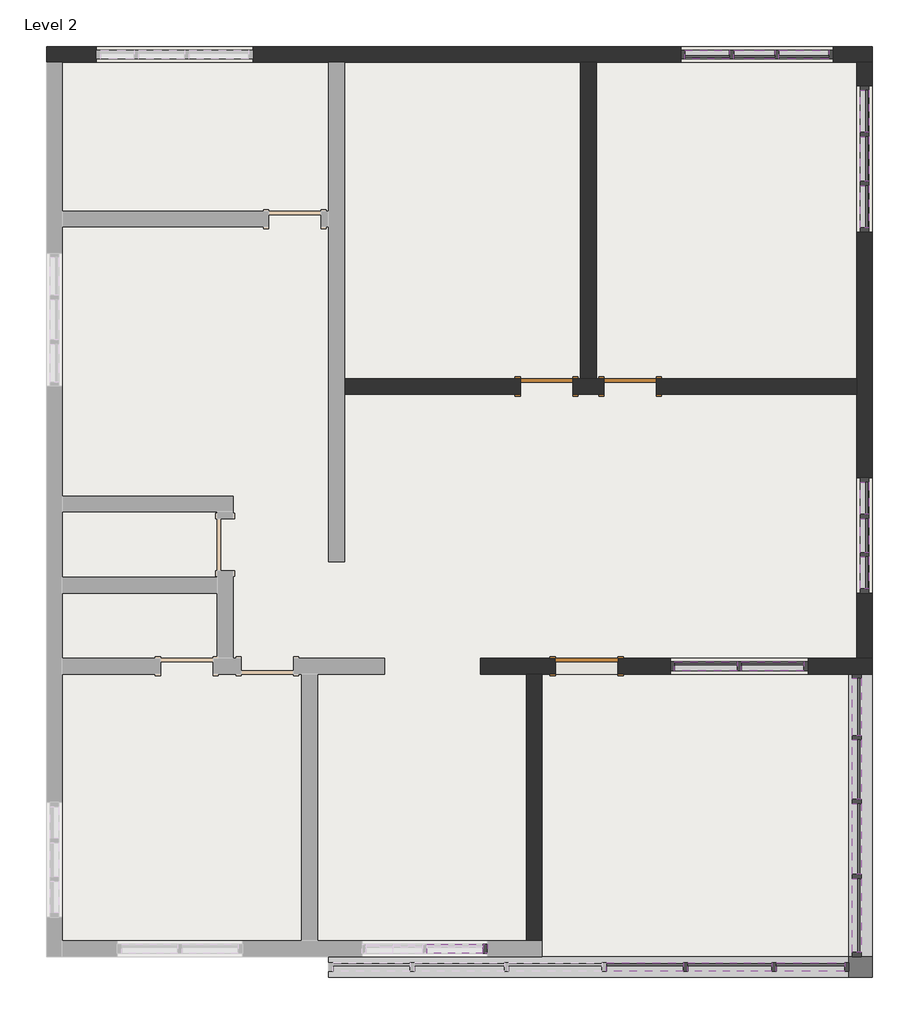
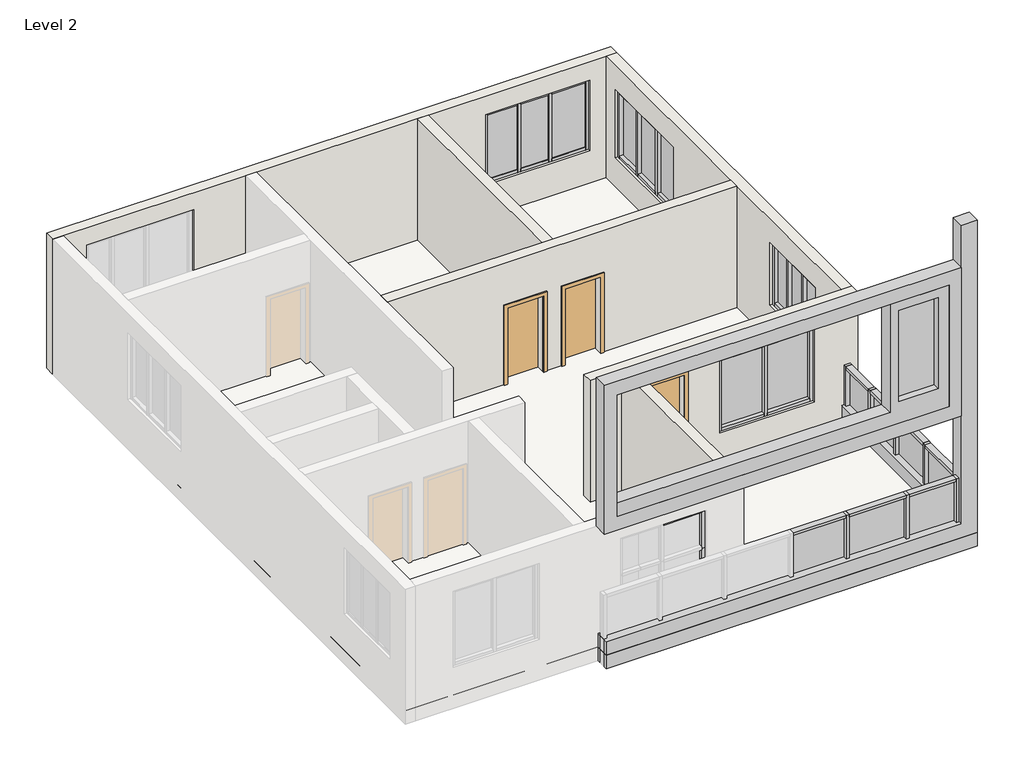
# One storey, part 2 of 2: 59 members, 18 plates, 6 walls, 3 doors, 2 proxies, 1 roof.
"""IFC4 building model written with IfcOpenShell, lengths in millimetres."""

from ifc_helpers import new_model, si_unit, frame, origin, place, context, project, spatial, polyline, outline, extrude, faceted_brep, transform, mapped, element, save
from components import generic_models_2_generic_models_2_cc0d390d, generic_models_3_generic_models_3_7314e451, door_a1484949, door_85036156, door_a90ba1ad, member_3f0e0172, member_5215b92c, member_61359a5b, member_c17f1be2, member_5535eeb3, member_2ebf4a73, member_0bf31a60, member_647c50ce, member_78a9872f, member_43b5e5be, member_a400357f, member_ea9411ea, member_8d44de84, member_42ca508f, member_8c3e4394, member_cac0d47b, member_4a65ca8f, member_0adfe7f4, member_001188f2, member_75b26f99, member_883d71fc, member_d722639b, member_62e0d4bf, member_79ceace6, member_4d6ef9b1, member_b70ee1cc, member_c5864796, member_66f327b8, member_a80f276a, system_panel_glazed_83e43f9b, system_panel_glazed_4ceb7c04, system_panel_glazed_bbfcf774, system_panel_glazed_f5702331, system_panel_glazed_135d4218, system_panel_glazed_d2b782c8, system_panel_glazed_c0907c48, system_panel_glazed_aa593011, system_panel_glazed_fc0c7c09, system_panel_glazed_9bd642df, system_panel_glazed_a16c717b, system_panel_glazed_1cb891c7, system_panel_glazed_caa91b16, system_panel_glazed_a6fb9a4f, system_panel_glazed_64bca335

model = new_model("IFC4")

# Units and contexts
model_context = context("Model", 3, world=origin())
ifc_project = project(units=[si_unit("LENGTHUNIT", "METRE", prefix="MILLI")], contexts=[model_context])

# Site, building, storey
site = spatial("IfcSite", under=ifc_project)
building = spatial("IfcBuilding", under=site)
storey = spatial("IfcBuildingStorey", under=building, Name="Level 2", Elevation=3048.0)

# Proxies
placement = place(None, origin())
generic_models_2_generic_models_2_shape = generic_models_2_generic_models_2_cc0d390d(model_context)
element("IfcBuildingElementProxy", 1, Name="Generic Models 2 : Generic Models 2", ObjectType="Generic Models 2 : Generic Models 2", at=placement, inside=storey, context=model_context, shape_type="MappedRepresentation", body=[
    mapped(generic_models_2_generic_models_2_shape, transform((0.0, 0.0, 0.0), x_axis=(1.0, 0.0, 0.0), y_axis=(0.0, 1.0, 0.0), z_axis=(0.0, 0.0, 1.0))),
])
generic_models_3_generic_models_3_shape = generic_models_3_generic_models_3_7314e451(model_context)
element("IfcBuildingElementProxy", 2, Name="Generic Models 3 : Generic Models 3", ObjectType="Generic Models 3 : Generic Models 3", at=placement, inside=storey, context=model_context, shape_type="MappedRepresentation", body=[
    mapped(generic_models_3_generic_models_3_shape, transform((0.0, 0.0, 0.0), x_axis=(1.0, 0.0, 0.0), y_axis=(0.0, 1.0, 0.0), z_axis=(0.0, 0.0, 1.0))),
])

# Doors
door_shape = door_a1484949(model_context)
element("IfcDoor", 3, ObjectType="Single-Flush : 30\" x 80\"", at=placement, inside=storey, context=model_context, shape_type="MappedRepresentation", body=[
    mapped(door_shape, transform((-12995.791855, -5548.3538163, 3048.0), x_axis=(1.0, 0.0, 0.0), y_axis=(0.0, 1.0, 0.0), z_axis=(0.0, 0.0, 1.0))),
])
door_2_shape = door_85036156(model_context)
element("IfcDoor", 4, ObjectType="Single-Flush : 30\" x 80\"", at=placement, inside=storey, context=model_context, shape_type="MappedRepresentation", body=[
    mapped(door_2_shape, transform((-11776.591855, -5548.3538163, 3048.0), x_axis=(-1.0, 0.0, 0.0), y_axis=(0.0, -1.0, 0.0), z_axis=(0.0, 0.0, 1.0))),
])
door_3_shape = door_a90ba1ad(model_context)
element("IfcDoor", 5, ObjectType="Single-Flush : 36\" x 84\"", at=placement, inside=storey, context=model_context, shape_type="MappedRepresentation", body=[
    mapped(door_3_shape, transform((-12411.591855, -9625.0538163, 3403.6), x_axis=(-1.0, 0.0, 0.0), y_axis=(0.0, -1.0, 0.0), z_axis=(0.0, 0.0, 1.0))),
])

# Members
member_shape = member_3f0e0172(model_context)
element("IfcMember", 6, ObjectType="Rectangular Mullion : 2.5\" x 5\" rectangular", at=placement, inside=storey, context=model_context, shape_type="MappedRepresentation", body=[
    mapped(member_shape, transform((-8360.291855, -2621.0038163, 4007.4850468), x_axis=(0.0, 0.0, -1.0), y_axis=(-1.0, 0.0, 0.0), z_axis=(0.0, 1.0, 0.0))),
])
element("IfcMember", 7, ObjectType="Rectangular Mullion : 2.5\" x 5\" rectangular", at=placement, inside=storey, context=model_context, shape_type="MappedRepresentation", body=[
    mapped(member_shape, transform((-8360.291855, -1230.3538163, 4007.4850468), x_axis=(0.0, 0.0, -1.0), y_axis=(-1.0, 0.0, 0.0), z_axis=(0.0, 1.0, 0.0))),
])
member_2_shape = member_5215b92c(model_context)
element("IfcMember", 8, ObjectType="Rectangular Mullion : 2.5\" x 5\" rectangular", at=placement, inside=storey, context=model_context, shape_type="MappedRepresentation", body=[
    mapped(member_2_shape, transform((-8360.291855, -1909.8038163, 4007.4850468), x_axis=(0.0, 0.0, -1.0), y_axis=(-1.0, 0.0, 0.0), z_axis=(0.0, 1.0, 0.0))),
])
element("IfcMember", 9, ObjectType="Rectangular Mullion : 2.5\" x 5\" rectangular", at=placement, inside=storey, context=model_context, shape_type="MappedRepresentation", body=[
    mapped(member_2_shape, transform((-8360.291855, -2557.5038163, 5545.6790625), x_axis=(0.0, 0.0, 1.0), y_axis=(-1.0, 0.0, 0.0), z_axis=(0.0, -1.0, 0.0))),
])
element("IfcMember", 10, ObjectType="Rectangular Mullion : 2.5\" x 5\" rectangular", at=placement, inside=storey, context=model_context, shape_type="MappedRepresentation", body=[
    mapped(member_shape, transform((-8360.291855, -1846.3038163, 5545.6790625), x_axis=(0.0, 0.0, 1.0), y_axis=(-1.0, 0.0, 0.0), z_axis=(0.0, -1.0, 0.0))),
])
element("IfcMember", 11, ObjectType="Rectangular Mullion : 2.5\" x 5\" rectangular", at=placement, inside=storey, context=model_context, shape_type="MappedRepresentation", body=[
    mapped(member_shape, transform((-8360.291855, -3236.9538163, 5545.6790625), x_axis=(0.0, 0.0, 1.0), y_axis=(-1.0, 0.0, 0.0), z_axis=(0.0, -1.0, 0.0))),
])
member_3_shape = member_61359a5b(model_context)
element("IfcMember", 12, ObjectType="Rectangular Mullion : 2.5\" x 5\" rectangular", at=placement, inside=storey, context=model_context, shape_type="MappedRepresentation", body=[
    mapped(member_3_shape, transform((-10976.491855, -709.6538163, 5669.9128008), x_axis=(0.0, 0.0, 1.0), y_axis=(0.0, 1.0, 0.0), z_axis=(-1.0, 0.0, 0.0))),
])
element("IfcMember", 13, ObjectType="Rectangular Mullion : 2.5\" x 5\" rectangular", at=placement, inside=storey, context=model_context, shape_type="MappedRepresentation", body=[
    mapped(member_3_shape, transform((-10330.9085217, -709.6538163, 4085.5528144), x_axis=(0.0, 0.0, -1.0), y_axis=(0.0, 1.0, 0.0), z_axis=(1.0, 0.0, 0.0))),
])
member_4_shape = member_c17f1be2(model_context)
element("IfcMember", 14, ObjectType="Rectangular Mullion : 2.5\" x 5\" rectangular", at=placement, inside=storey, context=model_context, shape_type="MappedRepresentation", body=[
    mapped(member_4_shape, transform((-13922.891855, -13739.8538163, 5631.310527), x_axis=(0.0, 0.0, 1.0), y_axis=(0.0, -1.0, 0.0), z_axis=(1.0, 0.0, 0.0))),
])
member_5_shape = member_5535eeb3(model_context)
element("IfcMember", 15, ObjectType="Rectangular Mullion : 2.5\" x 5\" rectangular", at=placement, inside=storey, context=model_context, shape_type="MappedRepresentation", body=[
    mapped(member_5_shape, transform((-8360.291855, -7408.9038163, 5557.0770518), x_axis=(0.0, 0.0, 1.0), y_axis=(-1.0, 0.0, 0.0), z_axis=(0.0, -1.0, 0.0))),
])
element("IfcMember", 16, ObjectType="Rectangular Mullion : 2.5\" x 5\" rectangular", at=placement, inside=storey, context=model_context, shape_type="MappedRepresentation", body=[
    mapped(member_5_shape, transform((-8360.291855, -8494.7538163, 5557.0770518), x_axis=(0.0, 0.0, 1.0), y_axis=(-1.0, 0.0, 0.0), z_axis=(0.0, -1.0, 0.0))),
])
member_6_shape = member_2ebf4a73(model_context)
element("IfcMember", 17, ObjectType="Rectangular Mullion : 2.5\" x 5\" rectangular", at=placement, inside=storey, context=model_context, shape_type="MappedRepresentation", body=[
    mapped(member_6_shape, transform((-8360.291855, -7967.7038163, 5557.0770518), x_axis=(0.0, 0.0, 1.0), y_axis=(-1.0, 0.0, 0.0), z_axis=(0.0, -1.0, 0.0))),
])
member_7_shape = member_0bf31a60(model_context)
element("IfcMember", 18, ObjectType="Rectangular Mullion : 2.5\" x 5\" rectangular", at=placement, inside=storey, context=model_context, shape_type="MappedRepresentation", body=[
    mapped(member_7_shape, transform((-8360.291855, -7440.6538163, 4148.8893788), x_axis=(0.0, -1.0, 0.0), y_axis=(-1.0, 0.0, 0.0), z_axis=(0.0, 0.0, -1.0))),
])
element("IfcMember", 19, ObjectType="Rectangular Mullion : 2.5\" x 5\" rectangular", at=placement, inside=storey, context=model_context, shape_type="MappedRepresentation", body=[
    mapped(member_7_shape, transform((-8360.291855, -7999.4538163, 4148.8893788), x_axis=(0.0, -1.0, 0.0), y_axis=(-1.0, 0.0, 0.0), z_axis=(0.0, 0.0, -1.0))),
])
element("IfcMember", 20, ObjectType="Rectangular Mullion : 2.5\" x 5\" rectangular", at=placement, inside=storey, context=model_context, shape_type="MappedRepresentation", body=[
    mapped(member_6_shape, transform((-8360.291855, -7472.4038163, 4148.8893788), x_axis=(0.0, 0.0, -1.0), y_axis=(-1.0, 0.0, 0.0), z_axis=(0.0, 1.0, 0.0))),
])
element("IfcMember", 21, ObjectType="Rectangular Mullion : 2.5\" x 5\" rectangular", at=placement, inside=storey, context=model_context, shape_type="MappedRepresentation", body=[
    mapped(member_5_shape, transform((-8360.291855, -8031.2038163, 4148.8893788), x_axis=(0.0, 0.0, -1.0), y_axis=(-1.0, 0.0, 0.0), z_axis=(0.0, 1.0, 0.0))),
])
element("IfcMember", 22, ObjectType="Rectangular Mullion : 2.5\" x 5\" rectangular", at=placement, inside=storey, context=model_context, shape_type="MappedRepresentation", body=[
    mapped(member_5_shape, transform((-8360.291855, -6945.3538163, 4148.8893788), x_axis=(0.0, 0.0, -1.0), y_axis=(-1.0, 0.0, 0.0), z_axis=(0.0, 1.0, 0.0))),
])
member_8_shape = member_647c50ce(model_context)
element("IfcMember", 23, ObjectType="Rectangular Mullion : 2.5\" x 5\" rectangular", at=placement, inside=storey, context=model_context, shape_type="MappedRepresentation", body=[
    mapped(member_8_shape, transform((-8360.291855, -6881.8538163, 5557.0770518), x_axis=(0.0, 1.0, 0.0), y_axis=(-1.0, 0.0, 0.0), z_axis=(0.0, 0.0, 1.0))),
])
element("IfcMember", 24, ObjectType="Rectangular Mullion : 2.5\" x 5\" rectangular", at=placement, inside=storey, context=model_context, shape_type="MappedRepresentation", body=[
    mapped(member_8_shape, transform((-8360.291855, -8558.2538163, 4148.8893788), x_axis=(0.0, -1.0, 0.0), y_axis=(-1.0, 0.0, 0.0), z_axis=(0.0, 0.0, -1.0))),
])
member_9_shape = member_78a9872f(model_context)
element("IfcMember", 25, ObjectType="Rectangular Mullion : 2.5\" x 5\" rectangular", at=placement, inside=storey, context=model_context, shape_type="MappedRepresentation", body=[
    mapped(member_9_shape, transform((-8360.291855, -1878.0538163, 4007.4850468), x_axis=(0.0, -1.0, 0.0), y_axis=(-1.0, 0.0, 0.0), z_axis=(0.0, 0.0, -1.0))),
])
element("IfcMember", 26, ObjectType="Rectangular Mullion : 2.5\" x 5\" rectangular", at=placement, inside=storey, context=model_context, shape_type="MappedRepresentation", body=[
    mapped(member_9_shape, transform((-8360.291855, -2589.2538163, 4007.4850468), x_axis=(0.0, -1.0, 0.0), y_axis=(-1.0, 0.0, 0.0), z_axis=(0.0, 0.0, -1.0))),
])
member_10_shape = member_43b5e5be(model_context)
element("IfcMember", 27, ObjectType="Rectangular Mullion : 2.5\" x 5\" rectangular", at=placement, inside=storey, context=model_context, shape_type="MappedRepresentation", body=[
    mapped(member_10_shape, transform((-8360.291855, -1166.8538163, 5545.6790625), x_axis=(0.0, 1.0, 0.0), y_axis=(-1.0, 0.0, 0.0), z_axis=(0.0, 0.0, 1.0))),
])
element("IfcMember", 28, ObjectType="Rectangular Mullion : 2.5\" x 5\" rectangular", at=placement, inside=storey, context=model_context, shape_type="MappedRepresentation", body=[
    mapped(member_10_shape, transform((-8360.291855, -3300.4538163, 4007.4850468), x_axis=(0.0, -1.0, 0.0), y_axis=(-1.0, 0.0, 0.0), z_axis=(0.0, 0.0, -1.0))),
])
member_11_shape = member_a400357f(model_context)
element("IfcMember", 29, ObjectType="Rectangular Mullion : 2.5\" x 5\" rectangular", at=placement, inside=storey, context=model_context, shape_type="MappedRepresentation", body=[
    mapped(member_11_shape, transform((-9670.5085217, -709.6538163, 4085.5528144), x_axis=(0.0, 0.0, -1.0), y_axis=(0.0, 1.0, 0.0), z_axis=(1.0, 0.0, 0.0))),
])
member_12_shape = member_ea9411ea(model_context)
element("IfcMember", 30, ObjectType="Rectangular Mullion : 2.5\" x 5\" rectangular", at=placement, inside=storey, context=model_context, shape_type="MappedRepresentation", body=[
    mapped(member_12_shape, transform((-8880.991855, -709.6538163, 4085.5528144), x_axis=(0.0, 0.0, -1.0), y_axis=(0.0, 1.0, 0.0), z_axis=(1.0, 0.0, 0.0))),
])
member_13_shape = member_8d44de84(model_context)
element("IfcMember", 31, ObjectType="Rectangular Mullion : 2.5\" x 5\" rectangular", at=placement, inside=storey, context=model_context, shape_type="MappedRepresentation", body=[
    mapped(member_13_shape, transform((-10299.1585217, -709.6538163, 4085.5528144), x_axis=(-1.0, 0.0, 0.0), y_axis=(0.0, 1.0, 0.0), z_axis=(0.0, 0.0, -1.0))),
])
element("IfcMember", 32, ObjectType="Rectangular Mullion : 2.5\" x 5\" rectangular", at=placement, inside=storey, context=model_context, shape_type="MappedRepresentation", body=[
    mapped(member_13_shape, transform((-9638.7585217, -709.6538163, 4085.5528144), x_axis=(-1.0, 0.0, 0.0), y_axis=(0.0, 1.0, 0.0), z_axis=(0.0, 0.0, -1.0))),
])
element("IfcMember", 33, ObjectType="Rectangular Mullion : 2.5\" x 5\" rectangular", at=placement, inside=storey, context=model_context, shape_type="MappedRepresentation", body=[
    mapped(member_12_shape, transform((-9607.0085217, -709.6538163, 5669.9128008), x_axis=(0.0, 0.0, 1.0), y_axis=(0.0, 1.0, 0.0), z_axis=(-1.0, 0.0, 0.0))),
])
element("IfcMember", 34, ObjectType="Rectangular Mullion : 2.5\" x 5\" rectangular", at=placement, inside=storey, context=model_context, shape_type="MappedRepresentation", body=[
    mapped(member_11_shape, transform((-10267.4085217, -709.6538163, 5669.9128008), x_axis=(0.0, 0.0, 1.0), y_axis=(0.0, 1.0, 0.0), z_axis=(-1.0, 0.0, 0.0))),
])
member_14_shape = member_42ca508f(model_context)
element("IfcMember", 35, ObjectType="Rectangular Mullion : 2.5\" x 5\" rectangular", at=placement, inside=storey, context=model_context, shape_type="MappedRepresentation", body=[
    mapped(member_14_shape, transform((-11039.991855, -709.6538163, 4085.5528144), x_axis=(-1.0, 0.0, 0.0), y_axis=(0.0, 1.0, 0.0), z_axis=(0.0, 0.0, -1.0))),
])
element("IfcMember", 36, ObjectType="Rectangular Mullion : 2.5\" x 5\" rectangular", at=placement, inside=storey, context=model_context, shape_type="MappedRepresentation", body=[
    mapped(member_14_shape, transform((-8817.491855, -709.6538163, 5669.9128008), x_axis=(1.0, 0.0, 0.0), y_axis=(0.0, 1.0, 0.0), z_axis=(0.0, 0.0, 1.0))),
])
member_15_shape = member_8c3e4394(model_context)
element("IfcMember", 37, ObjectType="Rectangular Mullion : 2.5\" x 5\" rectangular", at=placement, inside=storey, context=model_context, shape_type="MappedRepresentation", body=[
    mapped(member_15_shape, transform((-10217.666855, -9625.0538163, 5592.5131116), x_axis=(0.0, 0.0, 1.0), y_axis=(0.0, -1.0, 0.0), z_axis=(1.0, 0.0, 0.0))),
])
element("IfcMember", 38, ObjectType="Rectangular Mullion : 2.5\" x 5\" rectangular", at=placement, inside=storey, context=model_context, shape_type="MappedRepresentation", body=[
    mapped(member_15_shape, transform((-9242.941855, -9625.0538163, 5592.5131116), x_axis=(0.0, 0.0, 1.0), y_axis=(0.0, -1.0, 0.0), z_axis=(1.0, 0.0, 0.0))),
])
member_16_shape = member_cac0d47b(model_context)
element("IfcMember", 39, ObjectType="Rectangular Mullion : 2.5\" x 5\" rectangular", at=placement, inside=storey, context=model_context, shape_type="MappedRepresentation", body=[
    mapped(member_16_shape, transform((-10185.916855, -9625.0538163, 3942.9226891), x_axis=(1.0, 0.0, 0.0), y_axis=(0.0, -1.0, 0.0), z_axis=(0.0, 0.0, -1.0))),
])
element("IfcMember", 40, ObjectType="Rectangular Mullion : 2.5\" x 5\" rectangular", at=placement, inside=storey, context=model_context, shape_type="MappedRepresentation", body=[
    mapped(member_15_shape, transform((-10154.166855, -9625.0538163, 3942.9226891), x_axis=(0.0, 0.0, -1.0), y_axis=(0.0, -1.0, 0.0), z_axis=(-1.0, 0.0, 0.0))),
])
element("IfcMember", 41, ObjectType="Rectangular Mullion : 2.5\" x 5\" rectangular", at=placement, inside=storey, context=model_context, shape_type="MappedRepresentation", body=[
    mapped(member_15_shape, transform((-11128.891855, -9625.0538163, 3942.9226891), x_axis=(0.0, 0.0, -1.0), y_axis=(0.0, -1.0, 0.0), z_axis=(-1.0, 0.0, 0.0))),
])
member_17_shape = member_4a65ca8f(model_context)
element("IfcMember", 42, ObjectType="Rectangular Mullion : 2.5\" x 5\" rectangular", at=placement, inside=storey, context=model_context, shape_type="MappedRepresentation", body=[
    mapped(member_17_shape, transform((-9179.441855, -9625.0538163, 3942.9226891), x_axis=(1.0, 0.0, 0.0), y_axis=(0.0, -1.0, 0.0), z_axis=(0.0, 0.0, -1.0))),
])
element("IfcMember", 43, ObjectType="Rectangular Mullion : 2.5\" x 5\" rectangular", at=placement, inside=storey, context=model_context, shape_type="MappedRepresentation", body=[
    mapped(member_17_shape, transform((-11192.391855, -9625.0538163, 5592.5131116), x_axis=(-1.0, 0.0, 0.0), y_axis=(0.0, -1.0, 0.0), z_axis=(0.0, 0.0, 1.0))),
])
member_18_shape = member_0adfe7f4(model_context)
element("IfcMember", 44, ObjectType="Rectangular Mullion : 2.5\" x 5\" rectangular", at=placement, inside=storey, context=model_context, shape_type="MappedRepresentation", body=[
    mapped(member_18_shape, transform((-13859.391855, -13739.8538163, 4760.0253323), x_axis=(1.0, 0.0, 0.0), y_axis=(0.0, -1.0, 0.0), z_axis=(0.0, 0.0, -1.0))),
])
element("IfcMember", 45, ObjectType="Rectangular Mullion : 2.5\" x 5\" rectangular", at=placement, inside=storey, context=model_context, shape_type="MappedRepresentation", body=[
    mapped(member_18_shape, transform((-13859.391855, -13739.8538163, 3888.7401376), x_axis=(1.0, 0.0, 0.0), y_axis=(0.0, -1.0, 0.0), z_axis=(0.0, 0.0, -1.0))),
])
member_19_shape = member_001188f2(model_context)
element("IfcMember", 46, ObjectType="Rectangular Mullion : 2.5\" x 5\" rectangular", at=placement, inside=storey, context=model_context, shape_type="MappedRepresentation", body=[
    mapped(member_19_shape, transform((-9679.0607234, -14006.5538163, 3048.0), x_axis=(1.0, 0.0, 0.0), y_axis=(0.0, -1.0, 0.0), z_axis=(0.0, 0.0, -1.0))),
])
element("IfcMember", 47, ObjectType="Rectangular Mullion : 2.5\" x 5\" rectangular", at=placement, inside=storey, context=model_context, shape_type="MappedRepresentation", body=[
    mapped(member_19_shape, transform((-10967.3481445, -14006.5538163, 3048.0), x_axis=(1.0, 0.0, 0.0), y_axis=(0.0, -1.0, 0.0), z_axis=(0.0, 0.0, -1.0))),
])
member_20_shape = member_75b26f99(model_context)
element("IfcMember", 48, ObjectType="Rectangular Mullion : 2.5\" x 5\" rectangular", at=placement, inside=storey, context=model_context, shape_type="MappedRepresentation", body=[
    mapped(member_20_shape, transform((-8586.8607234, -14006.5538163, 3048.0), x_axis=(1.0, 0.0, 0.0), y_axis=(0.0, -1.0, 0.0), z_axis=(0.0, 0.0, -1.0))),
])
member_21_shape = member_883d71fc(model_context)
element("IfcMember", 49, ObjectType="Rectangular Mullion : 2.5\" x 5\" rectangular", at=placement, inside=storey, context=model_context, shape_type="MappedRepresentation", body=[
    mapped(member_21_shape, transform((-8650.3607234, -14006.5538163, 4647.2829369), x_axis=(0.0, 0.0, 1.0), y_axis=(0.0, -1.0, 0.0), z_axis=(1.0, 0.0, 0.0))),
])
member_22_shape = member_d722639b(model_context)
element("IfcMember", 50, ObjectType="Rectangular Mullion : 2.5\" x 5\" rectangular", at=placement, inside=storey, context=model_context, shape_type="MappedRepresentation", body=[
    mapped(member_22_shape, transform((-9710.8107234, -14006.5538163, 4647.2829369), x_axis=(0.0, 0.0, 1.0), y_axis=(0.0, -1.0, 0.0), z_axis=(1.0, 0.0, 0.0))),
])
member_23_shape = member_62e0d4bf(model_context)
element("IfcMember", 51, ObjectType="Rectangular Mullion : 2.5\" x 5\" rectangular", at=placement, inside=storey, context=model_context, shape_type="MappedRepresentation", body=[
    mapped(member_23_shape, transform((-10999.0981445, -14006.5538163, 4647.2829369), x_axis=(0.0, 0.0, 1.0), y_axis=(0.0, -1.0, 0.0), z_axis=(1.0, 0.0, 0.0))),
])
member_24_shape = member_79ceace6(model_context)
element("IfcMember", 52, ObjectType="Rectangular Mullion : 2.5\" x 5\" rectangular", at=placement, inside=storey, context=model_context, shape_type="MappedRepresentation", body=[
    mapped(member_24_shape, transform((-8474.591855, -11625.3038163, 3575.4206061), x_axis=(0.0, 0.0, -1.0), y_axis=(-1.0, 0.0, 0.0), z_axis=(0.0, 1.0, 0.0))),
])
member_25_shape = member_4d6ef9b1(model_context)
element("IfcMember", 53, ObjectType="Rectangular Mullion : 2.5\" x 5\" rectangular", at=placement, inside=storey, context=model_context, shape_type="MappedRepresentation", body=[
    mapped(member_25_shape, transform((-8474.591855, -12717.5038163, 3575.4206061), x_axis=(0.0, 0.0, -1.0), y_axis=(-1.0, 0.0, 0.0), z_axis=(0.0, 1.0, 0.0))),
])
member_26_shape = member_b70ee1cc(model_context)
element("IfcMember", 54, ObjectType="Rectangular Mullion : 2.5\" x 5\" rectangular", at=placement, inside=storey, context=model_context, shape_type="MappedRepresentation", body=[
    mapped(member_26_shape, transform((-8474.591855, -10698.2038163, 3575.4206061), x_axis=(0.0, 0.0, -1.0), y_axis=(-1.0, 0.0, 0.0), z_axis=(0.0, 1.0, 0.0))),
])
member_27_shape = member_c5864796(model_context)
element("IfcMember", 55, ObjectType="Rectangular Mullion : 2.5\" x 5\" rectangular", at=placement, inside=storey, context=model_context, shape_type="MappedRepresentation", body=[
    mapped(member_27_shape, transform((-8474.591855, -9802.8538163, 3575.4206061), x_axis=(0.0, 0.0, -1.0), y_axis=(-1.0, 0.0, 0.0), z_axis=(0.0, 1.0, 0.0))),
])
member_28_shape = member_66f327b8(model_context)
element("IfcMember", 56, ObjectType="Rectangular Mullion : 2.5\" x 5\" rectangular", at=placement, inside=storey, context=model_context, shape_type="MappedRepresentation", body=[
    mapped(member_28_shape, transform((-8474.591855, -12685.7538163, 3575.4206061), x_axis=(0.0, -1.0, 0.0), y_axis=(-1.0, 0.0, 0.0), z_axis=(0.0, 0.0, -1.0))),
])
element("IfcMember", 57, ObjectType="Rectangular Mullion : 2.5\" x 5\" rectangular", at=placement, inside=storey, context=model_context, shape_type="MappedRepresentation", body=[
    mapped(member_28_shape, transform((-8474.591855, -11593.5538163, 3575.4206061), x_axis=(0.0, -1.0, 0.0), y_axis=(-1.0, 0.0, 0.0), z_axis=(0.0, 0.0, -1.0))),
])
element("IfcMember", 58, ObjectType="Rectangular Mullion : 2.5\" x 5\" rectangular", at=placement, inside=storey, context=model_context, shape_type="MappedRepresentation", body=[
    mapped(member_28_shape, transform((-8474.591855, -10666.4538163, 3575.4206061), x_axis=(0.0, -1.0, 0.0), y_axis=(-1.0, 0.0, 0.0), z_axis=(0.0, 0.0, -1.0))),
])
element("IfcMember", 59, ObjectType="Rectangular Mullion : 2.5\" x 5\" rectangular", at=placement, inside=storey, context=model_context, shape_type="MappedRepresentation", body=[
    mapped(member_27_shape, transform((-8474.591855, -10634.7038163, 4555.4351711), x_axis=(0.0, 0.0, 1.0), y_axis=(-1.0, 0.0, 0.0), z_axis=(0.0, -1.0, 0.0))),
])
element("IfcMember", 60, ObjectType="Rectangular Mullion : 2.5\" x 5\" rectangular", at=placement, inside=storey, context=model_context, shape_type="MappedRepresentation", body=[
    mapped(member_26_shape, transform((-8474.591855, -11561.8038163, 4555.4351711), x_axis=(0.0, 0.0, 1.0), y_axis=(-1.0, 0.0, 0.0), z_axis=(0.0, -1.0, 0.0))),
])
element("IfcMember", 61, ObjectType="Rectangular Mullion : 2.5\" x 5\" rectangular", at=placement, inside=storey, context=model_context, shape_type="MappedRepresentation", body=[
    mapped(member_24_shape, transform((-8474.591855, -12654.0038163, 4555.4351711), x_axis=(0.0, 0.0, 1.0), y_axis=(-1.0, 0.0, 0.0), z_axis=(0.0, -1.0, 0.0))),
])
element("IfcMember", 62, ObjectType="Rectangular Mullion : 2.5\" x 5\" rectangular", at=placement, inside=storey, context=model_context, shape_type="MappedRepresentation", body=[
    mapped(member_25_shape, transform((-8474.591855, -13790.6538163, 4555.4351711), x_axis=(0.0, 0.0, 1.0), y_axis=(-1.0, 0.0, 0.0), z_axis=(0.0, -1.0, 0.0))),
])
member_29_shape = member_a80f276a(model_context)
element("IfcMember", 63, ObjectType="Rectangular Mullion : 2.5\" x 5\" rectangular", at=placement, inside=storey, context=model_context, shape_type="MappedRepresentation", body=[
    mapped(member_29_shape, transform((-8474.591855, -13854.1538163, 3575.4206061), x_axis=(0.0, -1.0, 0.0), y_axis=(-1.0, 0.0, 0.0), z_axis=(0.0, 0.0, -1.0))),
])
element("IfcMember", 64, ObjectType="Rectangular Mullion : 2.5\" x 5\" rectangular", at=placement, inside=storey, context=model_context, shape_type="MappedRepresentation", body=[
    mapped(member_29_shape, transform((-8474.591855, -9739.3538163, 4555.4351711), x_axis=(0.0, 1.0, 0.0), y_axis=(-1.0, 0.0, 0.0), z_axis=(0.0, 0.0, 1.0))),
])

# Plates
system_panel_glazed_shape = system_panel_glazed_83e43f9b(model_context)
element("IfcPlate", 65, ObjectType="System Panel : Glazed", at=placement, inside=storey, context=model_context, shape_type="MappedRepresentation", body=[
    mapped(system_panel_glazed_shape, transform((-8360.291855, -7177.1288163, 4212.3893788), x_axis=(0.0, -1.0, 0.0), y_axis=(1.0, 0.0, 0.0), z_axis=(0.0, 0.0, 1.0))),
])
element("IfcPlate", 66, ObjectType="System Panel : Glazed", at=placement, inside=storey, context=model_context, shape_type="MappedRepresentation", body=[
    mapped(system_panel_glazed_shape, transform((-8360.291855, -8262.9788163, 4212.3893788), x_axis=(0.0, -1.0, 0.0), y_axis=(1.0, 0.0, 0.0), z_axis=(0.0, 0.0, 1.0))),
])
system_panel_glazed_2_shape = system_panel_glazed_4ceb7c04(model_context)
element("IfcPlate", 67, ObjectType="System Panel : Glazed", at=placement, inside=storey, context=model_context, shape_type="MappedRepresentation", body=[
    mapped(system_panel_glazed_2_shape, transform((-8360.291855, -7720.0538163, 4212.3893788), x_axis=(0.0, -1.0, 0.0), y_axis=(1.0, 0.0, 0.0), z_axis=(0.0, 0.0, 1.0))),
])
system_panel_glazed_3_shape = system_panel_glazed_bbfcf774(model_context)
element("IfcPlate", 68, ObjectType="System Panel : Glazed", at=placement, inside=storey, context=model_context, shape_type="MappedRepresentation", body=[
    mapped(system_panel_glazed_3_shape, transform((-8360.291855, -1538.3288163, 4070.9850468), x_axis=(0.0, -1.0, 0.0), y_axis=(1.0, 0.0, 0.0), z_axis=(0.0, 0.0, 1.0))),
])
element("IfcPlate", 69, ObjectType="System Panel : Glazed", at=placement, inside=storey, context=model_context, shape_type="MappedRepresentation", body=[
    mapped(system_panel_glazed_3_shape, transform((-8360.291855, -2928.9788163, 4070.9850468), x_axis=(0.0, -1.0, 0.0), y_axis=(1.0, 0.0, 0.0), z_axis=(0.0, 0.0, 1.0))),
])
system_panel_glazed_4_shape = system_panel_glazed_f5702331(model_context)
element("IfcPlate", 70, ObjectType="System Panel : Glazed", at=placement, inside=storey, context=model_context, shape_type="MappedRepresentation", body=[
    mapped(system_panel_glazed_4_shape, transform((-8360.291855, -2233.6538163, 4070.9850468), x_axis=(0.0, -1.0, 0.0), y_axis=(1.0, 0.0, 0.0), z_axis=(0.0, 0.0, 1.0))),
])
system_panel_glazed_5_shape = system_panel_glazed_135d4218(model_context)
element("IfcPlate", 71, ObjectType="System Panel : Glazed", at=placement, inside=storey, context=model_context, shape_type="MappedRepresentation", body=[
    mapped(system_panel_glazed_5_shape, transform((-9244.0001883, -709.6538163, 4149.0528144), x_axis=(-1.0, 0.0, 0.0), y_axis=(0.0, -1.0, 0.0), z_axis=(0.0, 0.0, 1.0))),
])
system_panel_glazed_6_shape = system_panel_glazed_d2b782c8(model_context)
element("IfcPlate", 72, ObjectType="System Panel : Glazed", at=placement, inside=storey, context=model_context, shape_type="MappedRepresentation", body=[
    mapped(system_panel_glazed_6_shape, transform((-10653.7001883, -709.6538163, 4149.0528144), x_axis=(-1.0, 0.0, 0.0), y_axis=(0.0, -1.0, 0.0), z_axis=(0.0, 0.0, 1.0))),
])
system_panel_glazed_7_shape = system_panel_glazed_c0907c48(model_context)
element("IfcPlate", 73, ObjectType="System Panel : Glazed", at=placement, inside=storey, context=model_context, shape_type="MappedRepresentation", body=[
    mapped(system_panel_glazed_7_shape, transform((-9968.9585217, -709.6538163, 4149.0528144), x_axis=(-1.0, 0.0, 0.0), y_axis=(0.0, -1.0, 0.0), z_axis=(0.0, 0.0, 1.0))),
])
system_panel_glazed_8_shape = system_panel_glazed_aa593011(model_context)
element("IfcPlate", 74, ObjectType="System Panel : Glazed", at=placement, inside=storey, context=model_context, shape_type="MappedRepresentation", body=[
    mapped(system_panel_glazed_8_shape, transform((-10673.279355, -9625.0538163, 4006.4226891), x_axis=(1.0, 0.0, 0.0), y_axis=(0.0, 1.0, 0.0), z_axis=(0.0, 0.0, 1.0))),
])
element("IfcPlate", 75, ObjectType="System Panel : Glazed", at=placement, inside=storey, context=model_context, shape_type="MappedRepresentation", body=[
    mapped(system_panel_glazed_8_shape, transform((-9698.554355, -9625.0538163, 4006.4226891), x_axis=(1.0, 0.0, 0.0), y_axis=(0.0, 1.0, 0.0), z_axis=(0.0, 0.0, 1.0))),
])
system_panel_glazed_9_shape = system_panel_glazed_fc0c7c09(model_context)
element("IfcPlate", 76, ObjectType="System Panel : Glazed", at=placement, inside=storey, context=model_context, shape_type="MappedRepresentation", body=[
    mapped(system_panel_glazed_9_shape, transform((-9148.8357234, -14006.5538163, 3048.0), x_axis=(1.0, 0.0, 0.0), y_axis=(0.0, 1.0, 0.0), z_axis=(0.0, 0.0, 1.0))),
])
system_panel_glazed_10_shape = system_panel_glazed_9bd642df(model_context)
element("IfcPlate", 77, ObjectType="System Panel : Glazed", at=placement, inside=storey, context=model_context, shape_type="MappedRepresentation", body=[
    mapped(system_panel_glazed_10_shape, transform((-11562.4699997, -14006.5538163, 3048.0), x_axis=(1.0, 0.0, 0.0), y_axis=(0.0, 1.0, 0.0), z_axis=(0.0, 0.0, 1.0))),
])
system_panel_glazed_11_shape = system_panel_glazed_a16c717b(model_context)
element("IfcPlate", 78, ObjectType="System Panel : Glazed", at=placement, inside=storey, context=model_context, shape_type="MappedRepresentation", body=[
    mapped(system_panel_glazed_11_shape, transform((-10323.2044339, -14006.5538163, 3048.0), x_axis=(1.0, 0.0, 0.0), y_axis=(0.0, 1.0, 0.0), z_axis=(0.0, 0.0, 1.0))),
])
system_panel_glazed_12_shape = system_panel_glazed_1cb891c7(model_context)
element("IfcPlate", 79, ObjectType="System Panel : Glazed", at=placement, inside=storey, context=model_context, shape_type="MappedRepresentation", body=[
    mapped(system_panel_glazed_12_shape, transform((-8474.591855, -10218.7788163, 3638.9206061), x_axis=(0.0, -1.0, 0.0), y_axis=(1.0, 0.0, 0.0), z_axis=(0.0, 0.0, 1.0))),
])
system_panel_glazed_13_shape = system_panel_glazed_caa91b16(model_context)
element("IfcPlate", 80, ObjectType="System Panel : Glazed", at=placement, inside=storey, context=model_context, shape_type="MappedRepresentation", body=[
    mapped(system_panel_glazed_13_shape, transform((-8474.591855, -13254.0788163, 3638.9206061), x_axis=(0.0, -1.0, 0.0), y_axis=(1.0, 0.0, 0.0), z_axis=(0.0, 0.0, 1.0))),
])
system_panel_glazed_14_shape = system_panel_glazed_a6fb9a4f(model_context)
element("IfcPlate", 81, ObjectType="System Panel : Glazed", at=placement, inside=storey, context=model_context, shape_type="MappedRepresentation", body=[
    mapped(system_panel_glazed_14_shape, transform((-8474.591855, -12139.6538163, 3638.9206061), x_axis=(0.0, -1.0, 0.0), y_axis=(1.0, 0.0, 0.0), z_axis=(0.0, 0.0, 1.0))),
])
system_panel_glazed_15_shape = system_panel_glazed_64bca335(model_context)
element("IfcPlate", 82, ObjectType="System Panel : Glazed", at=placement, inside=storey, context=model_context, shape_type="MappedRepresentation", body=[
    mapped(system_panel_glazed_15_shape, transform((-8474.591855, -11130.0038163, 3638.9206061), x_axis=(0.0, -1.0, 0.0), y_axis=(1.0, 0.0, 0.0), z_axis=(0.0, 0.0, 1.0))),
])

# Roof
element("IfcRoof", 83, ObjectType="Generic - 12\"", at=placement, inside=storey, context=model_context, shape_type="SweptSolid", body=[
    extrude(outline(polyline([(-20285.591855, -595.3538163), (-8245.991855, -595.3538163), (-8245.991855, -13854.1538163), (-20285.591855, -13854.1538163), (-20285.591855, -595.3538163)])), frame((0.0, 0.0, 3048.0), z_axis=(0.0, 0.0, 1.0), x_axis=(1.0, 0.0, 0.0)), (0.0, 0.0, 1.0), 304.8),
])

# Walls
element("IfcWall", 84, ObjectType="9\"", at=placement, inside=storey, context=model_context, shape_type="Brep", body=[
    faceted_brep([(-8245.991855, -595.3538163, 3048.0), (-20285.591855, -595.3538163, 3048.0), (-20285.591855, -595.3538163, 6096.0), (-8245.991855, -595.3538163, 6096.0), (-8817.491855, -595.3538163, 4085.5528144), (-8817.491855, -595.3538163, 5669.9128008), (-11039.991855, -595.3538163, 5669.9128008), (-11039.991855, -595.3538163, 4085.5528144), (-19561.691855, -595.3538163, 5710.0962507), (-19561.691855, -595.3538163, 4156.5855814), (-17275.691855, -595.3538163, 4156.5855814), (-17275.691855, -595.3538163, 5710.0962507), (-20285.591855, -823.9538163, 3048.0), (-20056.991855, -823.9538163, 3048.0), (-16170.791855, -823.9538163, 3048.0), (-15942.191855, -823.9538163, 3048.0), (-12500.491855, -823.9538163, 3048.0), (-12271.891855, -823.9538163, 3048.0), (-8474.591855, -823.9538163, 3048.0), (-8245.991855, -823.9538163, 3048.0), (-8245.991855, -823.9538163, 6096.0), (-8474.591855, -823.9538163, 6096.0), (-12271.891855, -823.9538163, 6096.0), (-12500.491855, -823.9538163, 6096.0), (-15942.191855, -823.9538163, 6096.0), (-16170.791855, -823.9538163, 6096.0), (-20056.991855, -823.9538163, 6096.0), (-20285.591855, -823.9538163, 6096.0), (-8817.491855, -823.9538163, 5669.9128008), (-8817.491855, -823.9538163, 4085.5528144), (-11039.991855, -823.9538163, 4085.5528144), (-11039.991855, -823.9538163, 5669.9128008), (-19561.691855, -823.9538163, 4156.5855814), (-19561.691855, -823.9538163, 5710.0962507), (-17275.691855, -823.9538163, 5710.0962507), (-17275.691855, -823.9538163, 4156.5855814)], [[[0, 1, 2, 3], [4, 5, 6, 7], [8, 9, 10, 11]], [[12, 13, 14, 15, 16, 17, 18, 19, 20, 21, 22, 23, 24, 25, 26, 27], [28, 29, 30, 31], [32, 33, 34, 35]], [[1, 0, 19, 18, 17, 16, 15, 14, 13, 12]], [[3, 2, 27, 26, 25, 24, 23, 22, 21, 20]], [[2, 1, 12, 27]], [[0, 3, 20, 19]], [[28, 5, 4, 29]], [[5, 28, 31, 6]], [[6, 31, 30, 7]], [[29, 4, 7, 30]], [[32, 9, 8, 33]], [[33, 8, 11, 34]], [[34, 11, 10, 35]], [[9, 32, 35, 10]]]),
])
element("IfcWall", 85, ObjectType="9\"", at=placement, inside=storey, context=model_context, shape_type="SweptSolid", body=[
    extrude(outline(polyline([(-13059.291855, -9739.3538163), (-13059.291855, -13625.5538163), (-13287.891855, -13625.5538163), (-13287.891855, -9739.3538163), (-13059.291855, -9739.3538163)])), frame((0.0, 0.0, 3048.0), z_axis=(0.0, 0.0, 1.0), x_axis=(1.0, 0.0, 0.0)), (0.0, 0.0, 1.0), 3048.0),
])
element("IfcWall", 86, ObjectType="9\"", at=placement, inside=storey, context=model_context, shape_type="Brep", body=[
    faceted_brep([(-13960.991855, -9739.3538163, 3048.0), (-13287.891855, -9739.3538163, 3048.0), (-13059.291855, -9739.3538163, 3048.0), (-8245.991855, -9739.3538163, 3048.0), (-8245.991855, -9739.3538163, 6096.0), (-13059.291855, -9739.3538163, 6096.0), (-13287.891855, -9739.3538163, 6096.0), (-13960.991855, -9739.3538163, 6096.0), (-11954.391855, -9739.3538163, 3403.6), (-12868.791855, -9739.3538163, 3403.6), (-12868.791855, -9739.3538163, 5537.2), (-11954.391855, -9739.3538163, 5537.2), (-11192.391855, -9739.3538163, 3942.9226891), (-11192.391855, -9739.3538163, 5592.5131116), (-9179.441855, -9739.3538163, 5592.5131116), (-9179.441855, -9739.3538163, 3942.9226891), (-8245.991855, -9510.7538163, 3048.0), (-8474.591855, -9510.7538163, 3048.0), (-13960.991855, -9510.7538163, 3048.0), (-13960.991855, -9510.7538163, 6096.0), (-8474.591855, -9510.7538163, 6096.0), (-8245.991855, -9510.7538163, 6096.0), (-12868.791855, -9510.7538163, 3403.6), (-11954.391855, -9510.7538163, 3403.6), (-11954.391855, -9510.7538163, 5537.2), (-12868.791855, -9510.7538163, 5537.2), (-11192.391855, -9510.7538163, 5592.5131116), (-11192.391855, -9510.7538163, 3942.9226891), (-9179.441855, -9510.7538163, 3942.9226891), (-9179.441855, -9510.7538163, 5592.5131116)], [[[0, 1, 2, 3, 4, 5, 6, 7], [8, 9, 10, 11], [12, 13, 14, 15]], [[16, 17, 18, 19, 20, 21], [22, 23, 24, 25], [26, 27, 28, 29]], [[3, 2, 1, 0, 18, 17, 16]], [[7, 6, 5, 4, 21, 20, 19]], [[0, 7, 19, 18]], [[4, 3, 16, 21]], [[9, 8, 23, 22]], [[10, 9, 22, 25]], [[11, 10, 25, 24]], [[8, 11, 24, 23]], [[12, 27, 26, 13]], [[13, 26, 29, 14]], [[14, 29, 28, 15]], [[27, 12, 15, 28]]]),
])
element("IfcWall", 87, ObjectType="9\"", at=placement, inside=storey, context=model_context, shape_type="Brep", body=[
    faceted_brep([(-8245.991855, -9510.7538163, 3048.0), (-8245.991855, -823.9538163, 3048.0), (-8245.991855, -823.9538163, 6096.0), (-8245.991855, -9510.7538163, 6096.0), (-8245.991855, -6881.8538163, 5557.0770518), (-8245.991855, -6881.8538163, 4148.8893788), (-8245.991855, -8558.2538163, 4148.8893788), (-8245.991855, -8558.2538163, 5557.0770518), (-8245.991855, -1166.8538163, 5545.6790625), (-8245.991855, -1166.8538163, 4007.4850468), (-8245.991855, -3300.4538163, 4007.4850468), (-8245.991855, -3300.4538163, 5545.6790625), (-8474.591855, -823.9538163, 3048.0), (-8474.591855, -5434.0538163, 3048.0), (-8474.591855, -5662.6538163, 3048.0), (-8474.591855, -9510.7538163, 3048.0), (-8474.591855, -9510.7538163, 6096.0), (-8474.591855, -5662.6538163, 6096.0), (-8474.591855, -5434.0538163, 6096.0), (-8474.591855, -823.9538163, 6096.0), (-8474.591855, -6881.8538163, 4148.8893788), (-8474.591855, -6881.8538163, 5557.0770518), (-8474.591855, -8558.2538163, 5557.0770518), (-8474.591855, -8558.2538163, 4148.8893788), (-8474.591855, -1166.8538163, 4007.4850468), (-8474.591855, -1166.8538163, 5545.6790625), (-8474.591855, -3300.4538163, 5545.6790625), (-8474.591855, -3300.4538163, 4007.4850468)], [[[0, 1, 2, 3], [4, 5, 6, 7], [8, 9, 10, 11]], [[12, 13, 14, 15, 16, 17, 18, 19], [20, 21, 22, 23], [24, 25, 26, 27]], [[1, 0, 15, 14, 13, 12]], [[3, 2, 19, 18, 17, 16]], [[2, 1, 12, 19]], [[0, 3, 16, 15]], [[20, 5, 4, 21]], [[21, 4, 7, 22]], [[22, 7, 6, 23]], [[5, 20, 23, 6]], [[24, 9, 8, 25]], [[25, 8, 11, 26]], [[10, 27, 26, 11]], [[9, 24, 27, 10]]]),
])
element("IfcWall", 88, ObjectType="9\"", at=placement, inside=storey, context=model_context, shape_type="Brep", body=[
    faceted_brep([(-12614.791855, -5662.6538163, 3048.0), (-12157.591855, -5662.6538163, 3048.0), (-12157.591855, -5662.6538163, 5080.0), (-11395.591855, -5662.6538163, 5080.0), (-11395.591855, -5662.6538163, 3048.0), (-8474.591855, -5662.6538163, 3048.0), (-8474.591855, -5662.6538163, 6096.0), (-15942.191855, -5662.6538163, 6096.0), (-15942.191855, -5662.6538163, 3048.0), (-13376.791855, -5662.6538163, 3048.0), (-13376.791855, -5662.6538163, 5080.0), (-12614.791855, -5662.6538163, 5080.0), (-12157.591855, -5434.0538163, 5080.0), (-12157.591855, -5434.0538163, 3048.0), (-12271.891855, -5434.0538163, 3048.0), (-12500.491855, -5434.0538163, 3048.0), (-12614.791855, -5434.0538163, 3048.0), (-12614.791855, -5434.0538163, 5080.0), (-13376.791855, -5434.0538163, 5080.0), (-13376.791855, -5434.0538163, 3048.0), (-15942.191855, -5434.0538163, 3048.0), (-15942.191855, -5434.0538163, 6096.0), (-12500.491855, -5434.0538163, 6096.0), (-12271.891855, -5434.0538163, 6096.0), (-8474.591855, -5434.0538163, 6096.0), (-8474.591855, -5434.0538163, 3048.0), (-11395.591855, -5434.0538163, 3048.0), (-11395.591855, -5434.0538163, 5080.0)], [[[0, 1, 2, 3, 4, 5, 6, 7, 8, 9, 10, 11]], [[12, 13, 14, 15, 16, 17, 18, 19, 20, 21, 22, 23, 24, 25, 26, 27]], [[9, 8, 20, 19]], [[26, 25, 5, 4]], [[16, 15, 14, 13, 1, 0]], [[7, 6, 24, 23, 22, 21]], [[6, 5, 25, 24]], [[8, 7, 21, 20]], [[17, 16, 0, 11]], [[18, 17, 11, 10]], [[19, 18, 10, 9]], [[2, 1, 13, 12]], [[3, 2, 12, 27]], [[4, 3, 27, 26]]]),
])
element("IfcWall", 89, ObjectType="9\"", at=placement, inside=storey, context=model_context, shape_type="SweptSolid", body=[
    extrude(outline(polyline([(-12500.491855, -5434.0538163), (-12500.491855, -823.9538163), (-12271.891855, -823.9538163), (-12271.891855, -5434.0538163), (-12500.491855, -5434.0538163)])), frame((0.0, 0.0, 3048.0), z_axis=(0.0, 0.0, 1.0), x_axis=(1.0, 0.0, 0.0)), (0.0, 0.0, 1.0), 3048.0),
])

save(model, "model.ifc")

# Revit data of these elements
# Type "Single-Flush : 30\" x 80\""
#   Type Mark = "5"
#   Construction Type Id = "MDOOR"
#   Assembly Code = "C1020"
#   Analytic Construction = "Metal"
#   Thickness = 0' - 2"
#   Heat Transfer Coefficient (U) = 0.651978 BTU/(h·ft²·°F)
#   Height = 6' - 8"
#   Trim Projection Ext = 0' - 1"
#   Trim Projection Int = 0' - 1"
#   Trim Width = 0' - 3"
#   Width = 2' - 6"
#   Define Thermal Properties by = 1
#   Define Thermal Properties by = 1
#   Door Material = Door - Panel
#   Frame Material = Door - Frame
#   Visual Light Transmittance = 0
#   Solar Heat Gain Coefficient = 0
#   Function = (empty or 0)
#   Wall Closure = (empty or 0)
# Type "Single-Flush : 36\" x 84\""
#   Type Mark = "1"
#   Construction Type Id = "MDOOR"
#   Assembly Code = "C1020"
#   Analytic Construction = "Metal"
#   Thickness = 0' - 2"
#   Heat Transfer Coefficient (U) = 0.651978 BTU/(h·ft²·°F)
#   Height = 7' - 0"
#   Trim Projection Ext = 0' - 1"
#   Trim Projection Int = 0' - 1"
#   Trim Width = 0' - 3"
#   Width = 3' - 0"
#   Define Thermal Properties by = 1
#   Define Thermal Properties by = 1
#   Door Material = Door - Panel
#   Frame Material = Door - Frame
#   Visual Light Transmittance = 0
#   Solar Heat Gain Coefficient = 0
#   Function = (empty or 0)
#   Wall Closure = (empty or 0)
# Type "Rectangular Mullion : 2.5\" x 5\" rectangular"
#   built-in parameter 1007304 = 0.416667 (stored number, unit not read)
#   built-in parameter 1007301 = 0.104167 (stored number, unit not read)
#   built-in parameter 1007300 = 0.104167 (stored number, unit not read)
# Type "System Panel : Glazed"
#   Construction Type Id = "GSP4R"
#   Analytic Construction = "1/8 in Pilkington single glazing"
#   Visual Light Transmittance = 0.9
#   Solar Heat Gain Coefficient = 0.86
#   Heat Transfer Coefficient (U) = 1.18115 BTU/(h·ft²·°F)
#   Define Thermal Properties by = 1
# Type "Generic - 12\""
#   Assembly Code = "B1020"
#   Layers, outside or top first: 1' - 0" no material (function 1)
# Type "9\""
#   Assembly Code = "B2010"
#   Layers, outside or top first: 0' - 9" no material (function 1)
# Element 1 (IfcBuildingElementProxy, "Generic Models 2 : Generic Models 2")
#   Phase Created = New Construction
# Element 2 (IfcBuildingElementProxy, "Generic Models 3 : Generic Models 3")
#   Phase Created = New Construction
# Elements 3, 4 (IfcDoor, "Single-Flush : 30\" x 80\"")
#   Phase Created = New Construction
#   Materials on its faces: "Door - Frame", "Door - Panel"
# Element 5 (IfcDoor, "Single-Flush : 36\" x 84\"")
#   Phase Created = New Construction
#   Materials on its faces: "Door - Frame", "Door - Panel"
# Elements 6, 7, 8, 9, 10, 11, 12, 13, 14, 15, 16, 17, 18, 19, 20, 21, 22, 23, 24, 25, 26, 27, 28, 29, 30, 31, 32, 33, 34, 35, 36, 37, 38, 39, 40, 41, 42, 43, 44, 45, 46, 47, 48, 49, 50, 51, 52, 53, 54, 55, 56, 57, 58, 59, 60, 61, 62, 63, 64 (IfcMember, "Rectangular Mullion : 2.5\" x 5\" rectangular")
#   Phase Created = New Construction
#   Materials on its faces: "Aluminum"
# Elements 65, 66, 67, 68, 69, 70, 71, 72, 73, 74, 75, 76, 77, 78, 79, 80, 81, 82 (IfcPlate, "System Panel : Glazed")
#   Phase Created = New Construction
#   Materials on its faces: "Glass"
# Element 83 (IfcRoof, "Generic - 12\"")
#   built-in parameter 1001705 = 11 (stored number, unit not read)
#   built-in parameter 1001710 = 33615
#   Phase Created = New Construction
#   Materials on its faces: "Default Roof"
# Elements 84, 85, 86, 87, 88, 89 (IfcWall, "9\"")
#   Top Offset = 0' - 0"
#   Base Offset = 0' - 0"
#   Unconnected Height = 10' - 0"
#   wall height = 10' - 0"
#   Phase Created = New Construction
#   Base Constraint = Level 2
#   Materials on its faces: "Default Wall"
# Materials
#   "Door - Panel": class "Wood", colour RGB 210 159 95, transparency 0, Cost = 0
#   "Door - Frame": colour RGB 118 70 51, transparency 0, Cost = 0
#   "Aluminum": class "Metal", colour RGB 247 247 247, transparency 0, Description = "Aluminum 6061", Cost = 0
#   "Glass": class "Glass", colour RGB 0 128 192, transparency 0.75, Description = "Soda Lime Glass", Cost = 0
#   "Default Roof": colour RGB 88 101 114, transparency 0, Cost = 0
#   "Default Wall": colour RGB 128 128 128, transparency 0, Cost = 0
